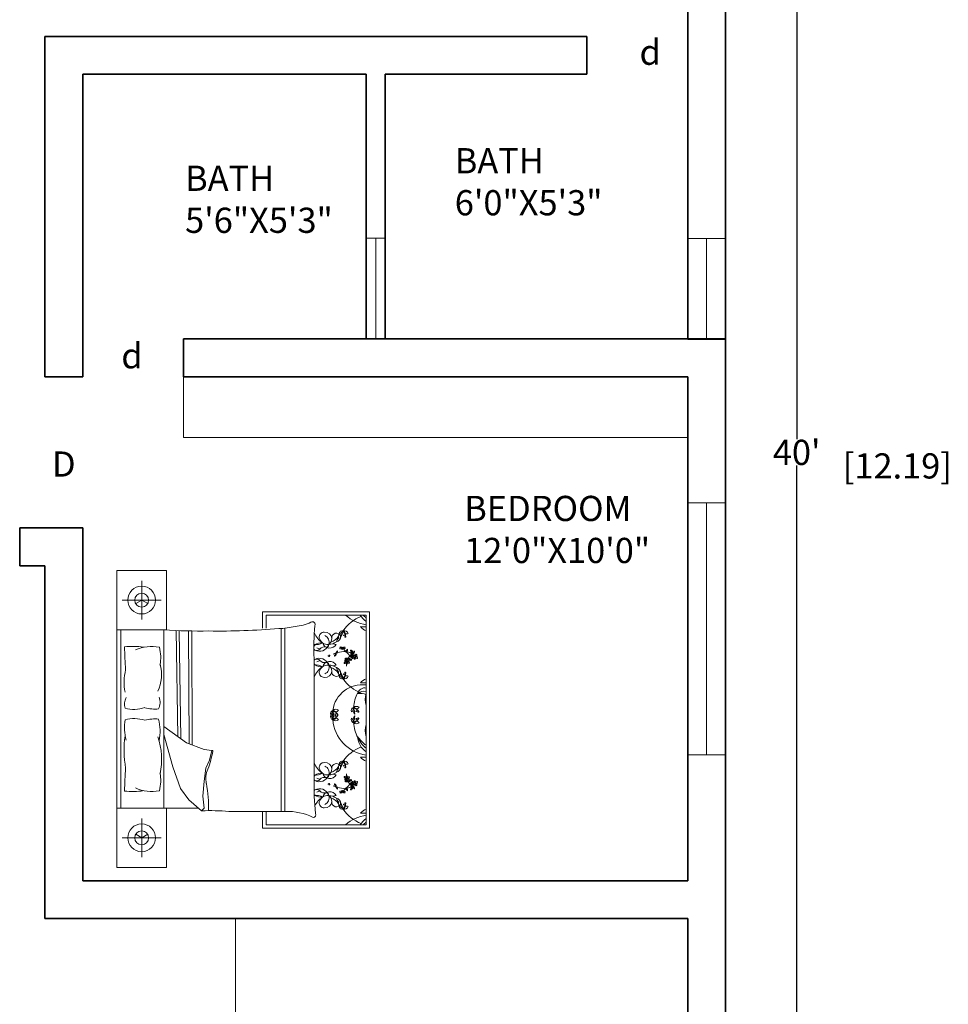
# Model space of a CAD drawing. Units: inches. Extents: x -43 to 1296, y -568 to 542.
# Tile 3 of 14: x 221 to 442, y -365 to -130. Entities that reach past the tile are written whole.
import ezdxf

# ---------------------------------------------------------------- set-up
doc = ezdxf.new("R2010")
doc.units = ezdxf.units.IN
doc.header["$MEASUREMENT"] = 0
for name, color, linetype, lineweight in [('A-ANNO-DIMS', 2, 'Continuous', 18), ('A-ANNO-TEXT', 7, 'Continuous', 18), ('A-AREA-IDEN', 7, 'Continuous', 18), ('A-FLOR-CASE', 9, 'Continuous', 18), ('A-FURN', 8, 'Continuous', 13), ('A-GLAZ', 6, 'Continuous', 18), ('A-WALL', 7, 'Continuous', 35)]:
    doc.layers.add(name, color=color, linetype=linetype, lineweight=lineweight)
doc.styles.get("Standard").update_dxf_attribs({"font": 'arial.ttf'})
doc.dimstyles.get("Standard").update_dxf_attribs({"dimtxt": 0.18, "dimasz": 0.18, "dimexe": 0.18, "dimexo": 0.0625, "dimgap": 0.09, "dimtad": 0, "dimtih": 1, "dimtoh": 1, "dimdec": 0, "dimzin": 0, "dimdsep": 46, "dimlunit": 3, "dimtxsty": 'Standard', "dimcen": 0.09, "dimadec": 0, "dimazin": 0, "dimtfac": 1, "dimtdec": 0, "dimtofl": 0, "dimtmove": 0, "dimatfit": 3, "dimfxl": 1, "dimtolj": 1, "dimtzin": 0, "dimarcsym": 0})

# ---------------------------------------------------------------- blocks, each defined once
blk = doc.blocks.new('*D2')
at = {"layer": 'A-ANNO-DIMS', "color": 0, "lineweight": -2, "transparency": 16777216}
for p, q in [((388.91, 6.66), (405.97, 6.66)), ((405.79, 6.48), (405.79, -230.19)), ((405.79, -473.16), (405.79, -236.49)), ((388.91, -473.34), (405.97, -473.34))]:
    blk.add_line(p, q, dxfattribs=at)
at = {"layer": 'A-ANNO-DIMS', "color": 0, "transparency": 16777216}
for points in [[(405.76, 6.48), (405.82, 6.48), (405.79, 6.66)], [(405.76, -473.16), (405.82, -473.16), (405.79, -473.34)]]:
    blk.add_solid(points, dxfattribs=at)
at = {"layer": 'Defpoints', "color": 0, "transparency": 16777216}
for p in [(388.84, 6.66), (388.84, -473.34), (405.79, -473.34)]:
    blk.add_point(p, dxfattribs=at)
at = {"layer": 'A-ANNO-DIMS', "color": 0, "transparency": 16777216, "insert": (405.79, -233.34), "char_height": 6, "attachment_point": 5}
blk.add_mtext("\\A1;40'", dxfattribs=at)
blk = doc.blocks.new('BED-SUITE-71')
for p, q in [((0, 0), (0, 70.73)), ((5.89, 59.04), (5.89, 68.28)), ((10.52, 63.66), (1.27, 63.66)), ((34.67, 56.98), (34.67, 60.9)), ((34.67, 60.9), (60.15, 60.9)), ((35.49, 60.08), (35.49, 56.97)), ((59.33, 60.08), (35.49, 60.08)), ((59.33, 10.16), (59.33, 60.08)), ((60.15, 60.9), (60.15, 9.34)), ((0.91, 56.59), (0.91, 14.15)), ((11.18, 14.15), (11.18, 56.59)), ((14.12, 56.4), (14.47, 31.21)), ((14.84, 56.37), (15.21, 30.69)), ((17.07, 56.33), (17.18, 29.47)), ((17.8, 56.34), (17.91, 29.2)), ((39.09, 56.91), (39.09, 13.33)), ((39.97, 56.97), (39.97, 13.33)), ((52.16, 53.11), (51.36, 53.27)), ((46.92, 49.73), (46.92, 21.01)), ((52.16, 48.17), (51.36, 48.01)), ((11.18, 33.58), (16.57, 29.7)), ((13.28, 23.97), (11.18, 31.68)), ((16.57, 29.7), (20.73, 28.13)), ((20.73, 28.13), (22.59, 27.84)), ((22.59, 27.84), (22.01, 25.55)), ((15.14, 18.81), (13.28, 23.97)), ((21.15, 23.69), (20.73, 20.53)), ((22.01, 25.55), (21.15, 23.69)), ((52.16, 22.07), (51.36, 22.23)), ((17.15, 16.09), (15.14, 18.81)), ((20.73, 20.53), (20.44, 16.95)), ((20.44, 16.95), (20.73, 14.09)), ((52.16, 17.13), (51.36, 16.97)), ((0, 14.15), (19.41, 14.15)), ((20.15, 13.51), (17.15, 16.09)), ((20.73, 14.09), (20.15, 13.51)), ((34.67, 9.34), (34.67, 13.34)), ((35.49, 13.34), (35.49, 10.16)), ((5.89, 11.69), (5.89, 2.45)), ((35.49, 10.16), (59.33, 10.16)), ((10.52, 7.07), (1.27, 7.07)), ((60.15, 9.34), (34.67, 9.34))]:
    blk.add_line(p, q)
for points in [[(0, 56.59), (11.79, 56.59), (11.79, 70.73), (0, 70.73)], [(5.89, 63.66), (4.47, 62.83)], [(5.89, 63.66), (7.32, 62.83)], [(11.79, 14.15), (11.79, 0), (0, 0)], [(5.89, 7.07), (4.47, 7.9)], [(5.89, 7.07), (7.32, 7.9)]]:
    blk.add_lwpolyline(points)
for points in [[(38.53, 56.89, 0.056112), (42.42, 57.4, 0.095341), (46.17, 58.4)], [(1.76, 52.52, -0.074897), (6.38, 52.44, 0.472817)], [(6.64, 38.06, -0.14099), (1.93, 37.91, -0.235245)], [(6.64, 35.04, 0.14099), (1.93, 35.18, 0.235245)], [(1.76, 18.21, 0.074897), (6.38, 18.3, -0.472817)], [(26.63, 13.37, 0.001242), (40.05, 13.33, -0.127202), (46.74, 11.91)]]:
    blk.add_lwpolyline(points, format="xyb")
for centre, radius in [((5.89, 63.66), 3.3), ((5.89, 63.66), 1.65), ((56.62, 50.21), 0.18), ((54.73, 49.03), 0.18), ((54.73, 21.21), 0.18), ((56.62, 20.03), 0.18), ((5.89, 7.07), 3.3), ((5.89, 7.07), 1.65)]:
    blk.add_circle(centre, radius)
for centre, radius, start, end in [((61.49, 51.16), 9.24, 111.4092, 145.6135), ((60.58, 66.96), 9.24, 228.1144, 262.255), ((61.82, 62.33), 4.5, 209.8884, 236.5383), ((62.65, 63.95), 5.61, 223.5186, 233.6964), ((19.82, 183.39), 127.09, 266.1, 270.9282), ((24.44, 222.08), 165.79, 269.1145, 274.8735), ((46.53, 57.86), 0.645, 336.5219, 123.8264), ((115.71, 51.89), 68.83, 175.2402, 181.8035), ((53.69, 55.63), 0.766, 76.272, 177.0484), ((52.52, 57.2), 1.58, 284.7031, 328.6173), ((54.72, 55.19), 1.46, 125.7657, 194.5347), ((47.56, 57.77), 6.46, 332.8176, 347.4827), ((54.09, 55.37), 1.02, 20.9613, 102.2885), ((54.64, 56.4), 0.771, 181.7131, 301.5367), ((52.11, 54.84), 2.34, 2.0648, 41.1598), ((53.52, 55.71), 0.756, 316.2238, 62.3173), ((60.77, 59.81), 3.76, 221.0454, 247.4453), ((58.76, 70.09), 12.78, 266.3481, 272.5919), ((51.9, 57.95), 5.35, 203.6453, 236.3329), ((49.33, 54.83), 1.19, 88.9462, 185.5144), ((50.21, 55.2), 2.13, 193.079, 274.7067), ((49.5, 54.34), 1.69, 7.1143, 95.0551), ((48.86, 53.68), 1.64, 338.5779, 68.4181), ((49.12, 54.64), 2.05, 305.9599, 357.6409), ((49.88, 56.84), 3.34, 288.2955, 328.7386), ((52.22, 54.73), 1.06, 19.1312, 189.736), ((51.9, 54.99), 1.33, 285.6955, 4.031), ((53.66, 53.56), 1.41, 128.4175, 173.8338), ((53.37, 54.95), 0.651, 126.7319, 206.0245), ((53.95, 55.26), 0.0602, 20.2667, 316.2271), ((54.27, 54.93), 0.0557, 52.0591, 168.5166), ((54.33, 54.92), 0.115, 168.5166, 2.0648), ((-671.38, 13.54), 674.27, 2.85022, 3.31479), ((8.24, 43.51), 9.12, 78.2417, 114.8684), ((0.94, 50), 9.48, 348.9631, 14.8961), ((47.7, 52.36), 0.852, 196.6343, 225.5483), ((47.44, 55.99), 2.93, 259.249, 301.1782), ((47.7, 52.36), 0.852, 127.675, 162.5814), ((48.2, 53.72), 2.25, 240.8249, 340.7178), ((47.53, 52.72), 1.06, 246.1646, 318.4347), ((48.71, 50.78), 2.73, 85.2696, 124.215), ((48.61, 54.06), 2.03, 240.0851, 262.564), ((49.41, 51.05), 1.45, 74.8529, 138.4347), ((50.64, 53.99), 1.76, 196.8663, 330.0915), ((49.9, 52.88), 0.439, 254.8529, 12.6959), ((48.71, 50.78), 2.73, 53.6555, 57.2989), ((50.15, 56.87), 3.8, 273.4924, 303.7117), ((53.16, 52.22), 0.139, 125.0752, 284.7644), ((53.38, 52.27), 0.3, 127.3642, 168.4363), ((53.14, 52.51), 0.433, 277.4968, 341.2737), ((53.48, 52.31), 0.172, 88.1325, 178.8919), ((53.83, 52.13), 0.372, 136.3462, 189.6513), ((53.62, 52.09), 0.155, 189.6513, 312.3208), ((53.66, 52.52), 0.18, 183.2768, 356.7232), ((54.22, 52.2), 0.59, 164.2829, 186.9148), ((53.52, 52.19), 0.295, 312.3208, 40.2111), ((54.15, 52.53), 0.419, 201.6382, 274.947), ((53.59, 51.95), 0.547, 42.3896, 66.5724), ((59.11, 56.28), 6.72, 217.9541, 226.8459), ((53.99, 52.27), 0.297, 10.9597, 52.2379), ((54.17, 52.25), 0.138, 274.947, 37.5263), ((54.64, 51.46), 0.144, 112.5583, 214.2343), ((54.54, 51.72), 0.339, 265.7131, 351.6568), ((54.24, 51.91), 0.593, 297.3659, 329.344), ((53.8, 52.42), 1.14, 313.6929, 321.7899), ((55.05, 51.64), 0.371, 115.5379, 168.6744), ((53.79, 52.18), 1.12, 329.344, 349.7412), ((52.9, 51.92), 1.99, 352.8698, 1.6736), ((55.7, 51.52), 0.201, 33.0979, 123.1364), ((51.27, 48.68), 5.26, 31.1156, 34.8118), ((55.41, 51.17), 0.545, 2.3172, 70.5201), ((55.62, 51.23), 0.469, 352.6008, 57.1845), ((47.7, 48.93), 0.852, 134.4517, 156.7144), ((48.2, 47.57), 2.25, 19.2822, 119.1751), ((47.53, 48.57), 1.06, 41.5653, 113.8354), ((48.61, 47.23), 2.03, 97.436, 119.9149), ((49.41, 50.23), 1.45, 221.5653, 285.1471), ((50.48, 50.45), 0.222, 169.5864, 349.5616), ((50.57, 50.44), 0.136, 349.5616, 167.2949), ((54.13, 45.54), 5.86, 110.1059, 116.9968), ((52.16, 50.36), 0.371, 129.5056, 182.6421), ((51.09, 51.22), 1.12, 308.4388, 328.836), ((50.9, 52.13), 1.99, 296.5064, 305.3102), ((50.88, 51.11), 1.14, 336.3901, 344.4871), ((52.12, 50.82), 0.144, 83.9457, 185.6216), ((51.54, 50.95), 0.593, 328.836, 0.8141), ((51.85, 50.78), 0.339, 306.5232, 32.4668), ((52.26, 51.04), 0.144, 112.5583, 214.2343), ((52.16, 51.3), 0.339, 265.7131, 351.6568), ((51.86, 51.49), 0.593, 297.3659, 329.344), ((51.42, 52), 1.14, 313.6929, 321.7899), ((52.67, 51.22), 0.371, 115.5379, 168.6744), ((51.41, 51.75), 1.12, 329.344, 349.7412), ((54.13, 45.54), 5.86, 86.1723, 106.4158), ((50.52, 51.5), 1.99, 352.8698, 1.6736), ((54.46, 50.41), 0.821, 253.6301, 325.4631), ((54.69, 49.27), 0.581, 82.0748, 142.6895), ((54.62, 50.06), 0.597, 228.342, 274.9894), ((54.41, 49.25), 0.176, 138.2946, 276.2474), ((54.48, 49.23), 0.246, 358.5719, 143.8954), ((54.62, 49.42), 0.248, 208.8493, 269.9355), ((54.27, 48.45), 2.94, 60.7959, 85.244), ((48.02, 44.23), 9.66, 37.8256, 47.7588), ((54.64, 49.97), 0.499, 273.8774, 357.1501), ((55.27, 49.07), 0.568, 121.9501, 165.2442), ((54.84, 50.32), 0.483, 262.0748, 308.2393), ((54.88, 49.29), 0.119, 262.868, 7.094), ((54.86, 49.39), 0.355, 278.5614, 22.5914), ((58.17, 48.15), 3.52, 156.1523, 156.9499), ((55.06, 49.41), 0.178, 44.3732, 121.9501), ((55.61, 49.82), 0.499, 181.4625, 249.4747), ((55.53, 50.22), 0.483, 215.1128, 261.2773), ((55.92, 50.19), 0.821, 197.889, 269.722), ((58.17, 48.15), 3.52, 130.182, 149.456), ((55.66, 49.91), 0.597, 248.3627, 295.0101), ((55.37, 49.17), 0.581, 20.6625, 81.2773), ((56.23, 50.16), 0.581, 139.3812, 199.9959), ((55.15, 50.58), 0.821, 310.9365, 22.7695), ((55.53, 50.53), 0.597, 285.6484, 332.2957), ((55.86, 51.04), 0.157, 135.7354, 318.1297), ((55.6, 51.29), 0.208, 315.7354, 31.1156), ((55.43, 50.85), 0.483, 319.3812, 5.5456), ((55.98, 51.04), 0.157, 68.2452, 250.6395), ((57.29, 48.08), 3.14, 111.7087, 116.2181), ((54.27, 48.45), 2.94, 47.5083, 55.9967), ((56.07, 51.34), 0.469, 252.8042, 349.6943), ((55.62, 50.5), 0.499, 331.1838, 51.6792), ((56.13, 49.9), 0.139, 125.0752, 284.7644), ((56.12, 51.38), 0.208, 248.2452, 323.6254), ((56.35, 49.96), 0.3, 93.635, 168.4363), ((55.93, 51.5), 0.545, 291.7087, 3.0299), ((56.31, 50.43), 0.176, 138.2946, 276.2474), ((56.11, 50.2), 0.433, 277.4968, 341.2737), ((56.37, 50.4), 0.246, 358.5719, 143.8954), ((52.05, 54.37), 5.26, 323.6254, 327.3216), ((56.45, 50), 0.172, 88.1325, 178.8919), ((56.52, 50.6), 0.248, 208.8493, 269.9355), ((56.31, 50.54), 0.283, 274.2123, 318.1587), ((56.8, 49.81), 0.372, 136.3462, 189.6513), ((56.59, 49.78), 0.155, 189.6513, 312.3208), ((56.36, 51.37), 0.201, 325.6077, 55.6462), ((57.19, 49.88), 0.59, 164.2829, 186.9148), ((57.17, 50.25), 0.568, 121.9501, 165.2442), ((56.49, 49.88), 0.295, 312.3208, 40.2111), ((57.12, 50.21), 0.419, 201.6382, 274.947), ((56.78, 50.47), 0.119, 262.868, 7.094), ((56.56, 49.64), 0.547, 42.3896, 66.5724), ((56.76, 50.57), 0.355, 278.5614, 22.5914), ((56.96, 49.96), 0.297, 10.9597, 118.7804), ((56.96, 50.58), 0.178, 44.3732, 121.9501), ((57.14, 49.93), 0.138, 274.947, 37.5263), ((14.14, 44.13), 12.43, 166.3427, 191.1841), ((1.63, 45.91), 9, 333.8761, 16.1746), ((47.7, 48.93), 0.852, 203.2856, 232.325), ((47.44, 45.3), 2.93, 58.8218, 100.2867), ((51.9, 43.33), 5.35, 123.6671, 158.5059), ((48.71, 50.51), 2.73, 235.785, 274.7304), ((50.21, 46.08), 2.13, 85.2933, 166.921), ((50.64, 47.29), 1.76, 29.9085, 163.1337), ((48.86, 47.61), 1.64, 291.5819, 21.4221), ((49.9, 48.41), 0.439, 347.3041, 105.1471), ((48.71, 50.51), 2.73, 302.7011, 306.3445), ((49.12, 46.65), 2.05, 2.3591, 54.0401), ((50.15, 44.42), 3.8, 56.2883, 86.5076), ((49.88, 44.45), 3.34, 31.2614, 71.7045), ((53.66, 47.73), 1.41, 186.1662, 231.5825), ((51.9, 46.3), 1.33, 355.969, 74.3045), ((54.23, 48.72), 0.139, 125.0752, 284.7644), ((54.45, 48.78), 0.3, 93.635, 168.4363), ((54.21, 49.02), 0.433, 277.4968, 341.2737), ((54.56, 48.82), 0.172, 88.1325, 178.8919), ((54.41, 49.36), 0.283, 274.2123, 318.1587), ((54.9, 48.63), 0.372, 136.3462, 189.6513), ((54.69, 48.6), 0.155, 189.6513, 312.3208), ((58.17, 48.15), 3.52, 175.2415, 182.8929), ((55.29, 48.7), 0.59, 164.2829, 186.9148), ((54.59, 48.7), 0.295, 312.3208, 40.2111), ((55.22, 49.03), 0.419, 201.6382, 274.947), ((54.66, 48.46), 0.547, 42.3896, 66.5724), ((55.06, 48.78), 0.297, 10.9597, 118.7804), ((55.24, 48.75), 0.138, 274.947, 37.5263), ((49.33, 46.45), 1.19, 174.4856, 271.0538), ((49.5, 46.94), 1.69, 264.9449, 352.8857), ((52.22, 46.55), 1.06, 170.264, 340.8688), ((53.37, 46.33), 0.651, 153.9755, 233.2681), ((53.69, 45.65), 0.766, 182.9516, 283.728), ((52.52, 44.09), 1.58, 31.3827, 75.2969), ((54.72, 46.09), 1.46, 165.4653, 234.2343), ((47.56, 43.51), 6.46, 12.5173, 27.1824), ((52.11, 46.45), 2.34, 318.8402, 357.9352), ((53.52, 45.58), 0.756, 297.6827, 43.7762), ((54.64, 44.89), 0.771, 58.4633, 178.2869), ((54.09, 45.91), 1.02, 257.7115, 339.0387), ((61.49, 50.13), 9.24, 214.3865, 248.5908), ((53.99, 46.03), 0.0999, 43.7762, 339.7183), ((54.33, 46.37), 0.115, 357.9352, 191.4834), ((54.27, 46.35), 0.0557, 191.4834, 307.9409), ((60.77, 41.48), 3.76, 112.5547, 138.9546), ((58.45, 36.38), 7.15, 82.8636, 171.8197), ((58.94, 41.1), 1.66, 76.3898, 169.0739), ((58.76, 31.19), 12.78, 87.4081, 93.6519), ((5.29, 38.88), 3.5, 153.3437, 196.1026), ((6.51, 39.36), 3.75, 335.0183, 18.5407), ((65.53, 37.39), 9.24, 152.5854, 175.5377), ((58.72, 39.85), 2.1, 72.8609, 131.9049), ((57.79, 37.31), 4.14, 68.117, 96.6195), ((64.19, 39.97), 5.08, 162.9798, 196.4569), ((9.01, 46.39), 8.67, 254.1707, 275.9871), ((52.06, 36.64), 1.02, 50.8855, 132.2127), ((56.53, 37.37), 0.766, 106.1963, 206.9726), ((54.74, 38.15), 1.58, 314.6273, 358.5415), ((57.65, 37.51), 1.46, 155.6899, 224.4589), ((57.01, 37.35), 1.02, 50.8855, 132.2127), ((56.97, 38.51), 0.771, 211.6373, 331.4609), ((55.56, 35.9), 2.34, 31.989, 71.0841), ((50.15, 36.17), 6.46, 2.7418, 17.407), ((56.35, 37.35), 0.756, 346.148, 92.2415), ((66.81, 37.96), 7.51, 174.3643, 175.6213), ((71.95, 34), 13.42, 160.0972, 160.2783), ((14.39, 33.32), 12.6, 171.5249, 193.96), ((9.01, 26.7), 8.67, 84.0129, 105.8293), ((-2.21, 32.38), 12.47, 349.8617, 13.6238), ((51.58, 36.66), 0.766, 106.1963, 206.9726), ((51.58, 35.93), 0.766, 153.0274, 253.8037), ((49.79, 37.44), 1.58, 314.6273, 358.5415), ((49.79, 35.16), 1.58, 1.4585, 45.3727), ((52.7, 36.8), 1.46, 155.6899, 224.4589), ((52.7, 35.8), 1.46, 135.5411, 204.3101), ((52.03, 37.8), 0.771, 211.6373, 331.4609), ((51.4, 36.64), 0.756, 346.148, 92.2415), ((50.61, 35.19), 2.34, 31.989, 71.0841), ((45.2, 35.47), 6.46, 2.7418, 17.407), ((45.2, 37.13), 6.46, 342.593, 357.2582), ((50.61, 37.41), 2.34, 288.9159, 328.011), ((51.4, 35.95), 0.756, 267.7585, 13.852), ((52.03, 34.79), 0.771, 28.5391, 148.3627), ((52.06, 35.96), 1.02, 227.7873, 309.1145), ((60.58, 35.92), 9.24, 184.4623, 262.255), ((52, 36.48), 0.0602, 50.1909, 346.0209), ((52.04, 36.11), 0.0999, 13.852, 309.9245), ((52.5, 36.37), 0.115, 198.4408, 31.989), ((52.44, 36.35), 0.0557, 81.9833, 198.4408), ((52.5, 36.23), 0.115, 328.011, 161.5592), ((52.44, 36.25), 0.0557, 161.5592, 278.0167), ((56.53, 35.23), 0.766, 153.0274, 253.8037), ((54.74, 34.45), 1.58, 1.4585, 45.3727), ((57.65, 35.09), 1.46, 135.5411, 204.3101), ((50.15, 36.42), 6.46, 342.593, 357.2582), ((55.56, 36.7), 2.34, 288.9159, 328.011), ((56.35, 35.25), 0.756, 267.7585, 13.852), ((56.94, 37.19), 0.0602, 50.1909, 346.0209), ((56.98, 35.4), 0.0999, 13.852, 309.9245), ((57.39, 37.05), 0.0557, 81.9833, 198.4408), ((57.39, 35.54), 0.0557, 161.5592, 278.0167), ((57.44, 37.07), 0.115, 198.4408, 31.989), ((57.44, 35.52), 0.115, 328.011, 161.5592), ((56.97, 34.09), 0.771, 28.5391, 148.3627), ((57.01, 35.25), 1.02, 227.7873, 309.1145), ((65.53, 35.21), 9.24, 184.4623, 207.4146), ((64.19, 32.63), 5.08, 163.5431, 197.0202), ((66.81, 34.64), 7.51, 184.3787, 185.6357), ((71.95, 38.59), 13.42, 199.7217, 199.9028), ((27.36, 27.9), 25.65, 172.2196, 189.497), ((-5.8, 25.72), 16.44, 348.0397, 19.2615), ((61.82, 31.28), 4.5, 181.272, 236.5383), ((64.23, 35.85), 8.34, 214.0123, 234.053), ((62.65, 32.9), 5.61, 197.8504, 233.6964), ((61.49, 20.11), 9.24, 111.4092, 145.6135), ((-4.14, 32.75), 27.43, 340.1194, 349.3383), ((22.64, 27.68), 0.171, 358.8623, 109.7536), ((58.76, 39.05), 12.78, 266.3481, 272.5919), ((60.77, 28.76), 3.76, 221.0454, 247.4453), ((-671.38, 57.2), 674.27, 356.68521, 357.14978), ((51.9, 26.91), 5.35, 201.4941, 236.3329), ((49.33, 23.79), 1.19, 88.9462, 185.5144), ((50.21, 24.15), 2.13, 193.079, 274.7067), ((49.5, 23.3), 1.69, 7.1143, 95.0551), ((48.86, 22.63), 1.64, 338.5779, 68.4181), ((49.12, 23.59), 2.05, 305.9599, 357.6409), ((49.88, 25.79), 3.34, 288.2955, 328.7386), ((52.22, 23.69), 1.06, 19.1312, 189.736), ((51.9, 23.94), 1.33, 285.6955, 4.031), ((53.66, 22.51), 1.41, 128.4175, 173.8338), ((53.37, 23.91), 0.651, 126.7319, 206.0245), ((53.69, 24.59), 0.766, 76.272, 177.0484), ((52.52, 26.15), 1.58, 284.7031, 328.6173), ((54.72, 24.15), 1.46, 125.7657, 194.5347), ((47.56, 26.73), 6.46, 332.8176, 347.4827), ((54.09, 24.33), 1.02, 20.9613, 102.2885), ((53.52, 24.66), 0.756, 316.2238, 62.3173), ((52.11, 23.79), 2.34, 2.0648, 41.1598), ((54.64, 25.35), 0.771, 181.7131, 301.5367), ((53.95, 24.22), 0.0602, 20.2667, 316.2271), ((54.27, 23.88), 0.0557, 52.0591, 168.5166), ((54.33, 23.87), 0.115, 168.5166, 2.0648), ((0.94, 20.73), 9.48, 345.1039, 11.0369), ((26.92, 21.1), 5.76, 156.2616, 191.3392), ((47.44, 24.94), 2.93, 259.7133, 301.1782), ((47.7, 21.31), 0.852, 127.675, 156.7144), ((48.2, 22.67), 2.25, 240.8249, 340.7178), ((48.71, 19.73), 2.73, 85.2696, 124.215), ((48.61, 23.01), 2.03, 240.0851, 262.564), ((49.41, 20.01), 1.45, 74.8529, 138.4347), ((50.64, 22.95), 1.76, 196.8663, 330.0915), ((49.9, 21.83), 0.439, 254.8529, 12.6959), ((48.71, 19.73), 2.73, 53.6555, 57.2989), ((50.15, 25.82), 3.8, 273.4924, 303.7117), ((54.23, 21.52), 0.139, 75.2356, 234.9248), ((54.45, 21.46), 0.3, 191.5637, 266.365), ((54.41, 20.99), 0.176, 83.7526, 221.7054), ((54.21, 21.22), 0.433, 18.7263, 82.5032), ((54.56, 21.42), 0.172, 181.1081, 271.8675), ((54.41, 20.88), 0.283, 41.8413, 85.7877), ((54.69, 21.64), 0.155, 47.6792, 170.3487), ((54.9, 21.61), 0.372, 170.3487, 223.6538), ((58.17, 22.09), 3.52, 177.1071, 184.7585), ((55.29, 21.53), 0.59, 173.0852, 195.7171), ((54.59, 21.54), 0.295, 319.7889, 47.6792), ((55.22, 21.21), 0.419, 85.053, 158.3618), ((54.66, 21.78), 0.547, 293.4276, 317.6104), ((55.06, 21.46), 0.297, 241.2196, 349.0403), ((54.86, 20.85), 0.355, 337.4086, 81.4386), ((55.24, 21.49), 0.138, 322.4737, 85.053), ((8.24, 27.22), 9.12, 245.1316, 281.7583), ((-4.9, 14.72), 26.7, 357.4519, 11.3392), ((120.54, 20.16), 73.63, 179.3433, 185.6887), ((47.7, 21.31), 0.852, 203.229, 225.5483), ((47.53, 21.67), 1.06, 246.1646, 318.4347), ((48.2, 16.52), 2.25, 19.2822, 119.1751), ((50.48, 19.79), 0.222, 10.4384, 190.4136), ((50.57, 19.8), 0.136, 192.7051, 10.4384), ((54.13, 24.7), 5.86, 243.0032, 249.8941), ((51.09, 19.02), 1.12, 31.164, 51.5612), ((52.16, 19.88), 0.371, 177.3579, 230.4944), ((50.9, 18.11), 1.99, 54.6898, 63.4936), ((50.88, 19.13), 1.14, 15.5129, 23.6099), ((52.12, 19.42), 0.144, 174.3784, 276.0543), ((51.85, 19.46), 0.339, 327.5332, 53.4768), ((51.54, 19.29), 0.593, 359.1859, 31.164), ((52.26, 19.2), 0.144, 145.7657, 247.4417), ((52.16, 18.94), 0.339, 8.3432, 94.2869), ((51.86, 18.75), 0.593, 30.656, 62.6341), ((51.42, 18.24), 1.14, 38.2101, 46.3071), ((52.67, 19.02), 0.371, 191.3256, 244.4621), ((51.41, 18.49), 1.12, 10.2588, 30.656), ((54.13, 24.7), 5.86, 253.5842, 273.8277), ((50.52, 18.74), 1.99, 358.3264, 7.1302), ((59.11, 13.96), 6.72, 133.1541, 142.0459), ((54.62, 20.18), 0.597, 85.0106, 131.658), ((54.46, 19.83), 0.821, 34.5369, 106.3699), ((54.69, 20.97), 0.581, 217.3105, 277.9252), ((54.48, 21.01), 0.246, 216.1046, 1.4281), ((54.62, 20.82), 0.248, 90.0645, 151.1507), ((54.64, 18.78), 0.144, 145.7657, 247.4417), ((48.02, 26.01), 9.66, 312.2412, 322.1744), ((54.27, 21.79), 2.94, 274.756, 299.2041), ((54.54, 18.52), 0.339, 8.3432, 94.2869), ((54.24, 18.33), 0.593, 30.656, 62.6341), ((54.64, 20.27), 0.499, 2.8499, 86.1226), ((55.27, 21.16), 0.568, 194.7558, 238.0499), ((54.84, 19.92), 0.483, 51.7607, 97.9252), ((54.88, 20.95), 0.119, 352.906, 97.132), ((58.17, 22.09), 3.52, 203.0501, 203.8477), ((55.06, 20.83), 0.178, 238.0499, 315.6268), ((55.61, 20.41), 0.499, 110.5253, 178.5375), ((55.92, 20.05), 0.821, 90.278, 162.111), ((55.53, 20.02), 0.483, 98.7227, 144.8872), ((58.17, 22.09), 3.52, 210.544, 229.818), ((55.66, 20.33), 0.597, 64.9899, 111.6373), ((55.37, 21.07), 0.581, 278.7227, 339.3375), ((55.41, 19.07), 0.545, 289.4799, 357.6828), ((51.27, 21.56), 5.26, 325.1882, 328.8844), ((56.23, 20.08), 0.581, 160.0041, 220.6188), ((55.15, 19.66), 0.821, 337.2305, 49.0635), ((55.53, 19.71), 0.597, 27.7043, 74.3516), ((55.86, 19.2), 0.157, 41.8703, 224.2646), ((55.6, 18.95), 0.208, 328.8844, 44.2646), ((55.43, 19.39), 0.483, 354.4544, 40.6188), ((55.98, 19.2), 0.157, 109.3605, 291.7548), ((55.62, 19.01), 0.469, 302.8155, 7.3992), ((57.29, 22.16), 3.14, 243.7819, 248.2913), ((54.27, 21.79), 2.94, 304.0033, 312.4917), ((55.62, 19.74), 0.499, 308.3208, 28.8162), ((56.07, 18.9), 0.469, 10.3057, 107.1958), ((56.13, 20.34), 0.139, 75.2356, 234.9248), ((56.12, 18.86), 0.208, 36.3746, 111.7548), ((56.35, 20.28), 0.3, 191.5637, 266.365), ((56.31, 19.81), 0.176, 83.7526, 221.7054), ((55.93, 18.74), 0.545, 356.9701, 68.2913), ((56.11, 20.04), 0.433, 18.7263, 82.5032), ((56.37, 19.84), 0.246, 216.1046, 1.4281), ((56.45, 20.24), 0.172, 181.1081, 271.8675), ((52.05, 15.87), 5.26, 32.6784, 36.3746), ((56.52, 19.64), 0.248, 90.0645, 151.1507), ((56.31, 19.7), 0.283, 41.8413, 85.7877), ((56.59, 20.46), 0.155, 47.6792, 170.3487), ((56.8, 20.43), 0.372, 170.3487, 223.6538), ((56.36, 18.87), 0.201, 304.3538, 34.3923), ((57.19, 20.36), 0.59, 173.0852, 195.7171), ((57.17, 19.99), 0.568, 194.7558, 238.0499), ((56.49, 20.36), 0.295, 319.7889, 47.6792), ((57.12, 20.03), 0.419, 85.053, 158.3618), ((56.78, 19.77), 0.119, 352.906, 97.132), ((56.56, 20.6), 0.547, 293.4276, 317.6104), ((56.96, 20.28), 0.297, 241.2196, 349.0403), ((56.76, 19.67), 0.355, 337.4086, 81.4386), ((56.96, 19.66), 0.178, 238.0499, 315.6268), ((57.14, 20.31), 0.138, 322.4737, 85.053), ((47.7, 17.88), 0.852, 134.4517, 153.558), ((47.7, 17.88), 0.852, 210.0293, 232.325), ((47.44, 14.25), 2.93, 58.8218, 99.1554), ((47.53, 17.52), 1.06, 41.5653, 113.8354), ((51.9, 12.29), 5.35, 123.6671, 153.2997), ((48.71, 19.46), 2.73, 235.785, 274.7304), ((48.61, 16.18), 2.03, 97.436, 119.9149), ((50.21, 15.04), 2.13, 85.2933, 166.921), ((49.41, 19.19), 1.45, 221.5653, 285.1471), ((50.64, 16.25), 1.76, 29.9085, 163.1337), ((48.86, 16.56), 1.64, 291.5819, 21.4221), ((49.9, 17.36), 0.439, 347.3041, 105.1471), ((48.71, 19.46), 2.73, 302.7011, 306.3445), ((49.12, 15.6), 2.05, 2.3591, 54.0401), ((50.15, 13.37), 3.8, 56.2883, 86.5076), ((49.88, 13.4), 3.34, 31.2614, 71.7045), ((51.9, 15.25), 1.33, 355.969, 74.3045), ((53.66, 16.68), 1.41, 186.1662, 231.5825), ((53.16, 18.02), 0.139, 75.2356, 234.9248), ((53.38, 17.97), 0.3, 191.5637, 232.6358), ((53.14, 17.73), 0.433, 18.7263, 82.5032), ((53.48, 17.93), 0.172, 181.1081, 271.8675), ((53.62, 18.15), 0.155, 47.6792, 170.3487), ((53.83, 18.11), 0.372, 170.3487, 223.6538), ((53.66, 17.72), 0.18, 3.2768, 176.7232), ((54.22, 18.04), 0.59, 173.0852, 195.7171), ((53.52, 18.05), 0.295, 319.7889, 47.6792), ((54.15, 17.71), 0.419, 85.053, 158.3618), ((53.59, 18.29), 0.547, 293.4276, 317.6104), ((53.99, 17.97), 0.297, 307.7621, 349.0403), ((54.17, 17.99), 0.138, 322.4737, 85.053), ((53.8, 17.82), 1.14, 38.2101, 46.3071), ((55.05, 18.6), 0.371, 191.3256, 244.4621), ((53.79, 18.06), 1.12, 10.2588, 30.656), ((52.9, 18.32), 1.99, 358.3264, 7.1302), ((55.7, 18.72), 0.201, 236.8636, 326.9021), ((49.33, 15.41), 1.19, 174.4856, 271.0538), ((49.5, 15.9), 1.69, 264.9449, 352.8857), ((52.22, 15.51), 1.06, 170.264, 340.8688), ((53.37, 15.29), 0.651, 153.9755, 233.2681), ((52.52, 13.04), 1.58, 31.3827, 75.2969), ((53.69, 14.61), 0.766, 182.9516, 283.728), ((54.72, 15.05), 1.46, 165.4653, 234.2343), ((47.56, 12.46), 6.46, 12.5173, 27.1824), ((52.11, 15.4), 2.34, 318.8402, 357.9352), ((53.52, 14.53), 0.756, 297.6827, 43.7762), ((54.64, 13.84), 0.771, 58.4633, 178.2869), ((54.09, 14.87), 1.02, 257.7115, 339.0387), ((53.99, 14.99), 0.0999, 43.7762, 339.7183), ((54.33, 15.32), 0.115, 357.9352, 191.4834), ((54.27, 15.31), 0.0557, 191.4834, 307.9409), ((21.91, -51.34), 64.88, 85.8294, 91.553), ((46.69, 12.56), 0.653, 273.98, 27.3412), ((61.49, 19.08), 9.24, 214.3865, 248.5908), ((60.58, 3.28), 9.24, 97.745, 131.8856), ((60.77, 10.43), 3.76, 112.5547, 138.9546), ((58.76, 0.15), 12.78, 87.4081, 93.6519), ((61.82, 7.91), 4.5, 123.4617, 150.1116), ((62.65, 6.29), 5.61, 126.3036, 136.4814)]:
    blk.add_arc(centre, radius, start, end)
blk = doc.blocks.new('WIN-60x9')
for p, q in [((0, 60), (0, 0)), ((9, 60), (0, 60)), ((4.5, 60), (4.5, 0)), ((9, 0), (9, 60)), ((0, 0), (9, 0))]:
    blk.add_line(p, q)
blk = doc.blocks.new('VENT-24x9')
for p, q in [((0, 0), (0, 24)), ((0, 24), (9, 24)), ((4.5, 24), (4.5, 0)), ((9, 24), (9, 0)), ((9, 0), (0, 0))]:
    blk.add_line(p, q)
blk = doc.blocks.new('VENT-24x4-5')
for p, q in [((4.5, 24), (0, 24)), ((0, 24), (0, 0)), ((2.25, 0), (2.25, 24)), ((4.5, 0), (4.5, 24)), ((0, 0), (4.5, 0))]:
    blk.add_line(p, q)

msp = doc.modelspace()

# ---------------------------------------------------------------- linework, layer by layer
at = {"layer": 'A-FLOR-CASE'}
for p, q in [((259.84, -215.34), (259.84, -229.82)), ((259.84, -229.82), (379.84, -229.82)), ((272.21, -344.34), (272.21, -371.34))]:
    msp.add_line(p, q, dxfattribs=at)
at = {"layer": 'A-WALL'}
for p, q in [((388.84, 6.66), (388.84, -473.34)), ((379.84, -2.34), (379.84, -206.34)), ((226.84, -134.34), (355.84, -134.34)), ((226.84, -134.34), (226.84, -215.34)), ((355.84, -143.34), (355.84, -134.34)), ((235.84, -143.34), (303.34, -143.34)), ((235.84, -143.34), (235.84, -215.34)), ((303.34, -143.34), (303.34, -206.34)), ((307.84, -143.34), (307.84, -206.34)), ((307.84, -143.34), (355.84, -143.34)), ((259.84, -206.34), (303.34, -206.34)), ((259.84, -206.34), (259.84, -215.34)), ((303.34, -206.34), (307.84, -206.34)), ((307.84, -206.34), (388.84, -206.34)), ((226.84, -215.34), (235.84, -215.34)), ((259.84, -215.34), (379.84, -215.34)), ((379.84, -215.34), (379.84, -335.34)), ((220.84, -251.34), (220.84, -260.34)), ((220.84, -251.34), (235.84, -251.34)), ((235.84, -251.34), (235.84, -335.34)), ((220.84, -260.34), (226.84, -260.34)), ((226.84, -260.34), (226.84, -344.34)), ((235.84, -335.34), (379.84, -335.34)), ((226.84, -344.34), (379.84, -344.34)), ((379.84, -344.34), (379.84, -464.34))]:
    msp.add_line(p, q, dxfattribs=at)

# ---------------------------------------------------------------- block references
at = {"layer": 'A-FURN'}
msp.add_blockref('BED-SUITE-71', (243.99, -332.17), dxfattribs=at)
at = {"layer": 'A-GLAZ'}
for name, p in [('VENT-24x4-5', (303.34, -206.34)), ('VENT-24x9', (379.84, -206.44)), ('WIN-60x9', (379.84, -305.34))]:
    msp.add_blockref(name, p, dxfattribs=at)

# ---------------------------------------------------------------- texts
at = {"layer": 'A-ANNO-DIMS', "insert": (416.76, -233.56), "char_height": 6, "attachment_point": 1}
msp.add_mtext('[12.19]', dxfattribs=at)
at = {"layer": 'A-ANNO-TEXT', "insert": (368.38, -135.08), "char_height": 6, "attachment_point": 1}
msp.add_mtext_dynamic_manual_height_columns('d', width=0.3471, gutter_width=1, heights=[0], dxfattribs=at)
at = {"layer": 'A-ANNO-TEXT', "char_height": 6, "attachment_point": 1}
for s, insert in [('d', (245.03, -207.34)), ('D', (228.53, -233.12))]:
    msp.add_mtext(s, dxfattribs=dict(at, insert=insert))
at = {"layer": 'A-AREA-IDEN', "char_height": 6, "attachment_point": 1}
for s, insert in [('BATH\\P6\'0"X5\'3"', (324.4, -160.91)), ('BATH\\P5\'6"X5\'3"', (260.21, -165.09)), ('BEDROOM\\P12\'0"X10\'0"', (326.65, -243.69))]:
    msp.add_mtext(s, dxfattribs=dict(at, insert=insert))

# ---------------------------------------------------------------- dimensions: what is measured, and where the dimension line sits
at = {"layer": 'A-ANNO-DIMS'}
dim = msp.add_linear_dim(base=(405.79, -473.34), p1=(388.84, 6.66), p2=(388.84, -473.34), angle=90, dimstyle='Standard', override={"dimtxt": 6, "dimclrd": 0, "dimclre": 0, "dimclrt": 0}, dxfattribs=at)
dim.commit()
dim.dimension.update_dxf_attribs({"geometry": '*D2', "text_midpoint": (405.79, -233.34)})

doc.saveas('drawing.dxf')
